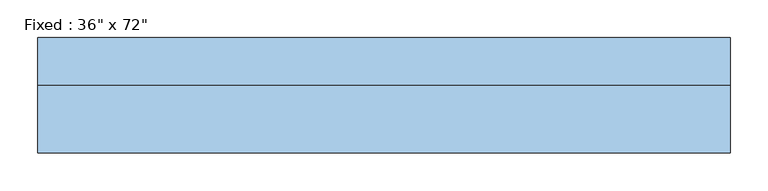
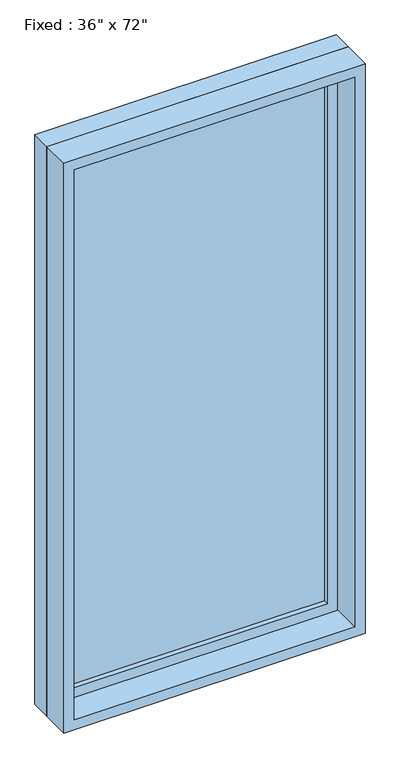
"""IFC4 building model written with IfcOpenShell, lengths in millimetres: window geometry."""

from ifc_helpers import new_model, si_unit, frame, origin, place, context, project, spatial, polyline, outline, extrude, source, transform, mapped, element, save


def window_c05a16fb(model_context):
    return source(origin(), model_context, "Body", "SweptSolid", [
        extrude(outline(polyline([(355.6, 28.575), (-431.8, 28.575), (-431.8, 41.275), (355.6, 41.275), (355.6, 28.575)])), frame((0.0, 0.0, 368.3), z_axis=(0.0, 0.0, 1.0), x_axis=(1.0, 0.0, 0.0)), (0.0, 0.0, 1.0), 1701.8),
        extrude(outline(polyline([(2114.55, -476.25), (323.85, -476.25), (323.85, 400.05), (2114.55, 400.05), (2114.55, -476.25)]), holes=[polyline([(2070.1, -431.8), (2070.1, 355.6), (368.3, 355.6), (368.3, -431.8), (2070.1, -431.8)])]), frame((0.0, 12.7, 0.0), z_axis=(0.0, 1.0, 0.0), x_axis=(0.0, 0.0, 1.0)), (0.0, 0.0, 1.0), 44.45),
        extrude(outline(polyline([(2133.6, -495.3), (304.8, -495.3), (304.8, 419.1), (2133.6, 419.1), (2133.6, -495.3)]), holes=[polyline([(2101.85, -463.55), (2101.85, 387.35), (336.55, 387.35), (336.55, -463.55), (2101.85, -463.55)])]), frame((0.0, -76.2, 0.0), z_axis=(0.0, 1.0, 0.0), x_axis=(0.0, 0.0, 1.0)), (0.0, 0.0, 1.0), 88.9),
        extrude(outline(polyline([(2133.6, 419.1), (2133.6, -495.3), (304.8, -495.3), (304.8, 419.1), (2133.6, 419.1)]), holes=[polyline([(2114.55, 400.05), (323.85, 400.05), (323.85, -476.25), (2114.55, -476.25), (2114.55, 400.05)])]), frame((0.0, 12.7, 0.0), z_axis=(0.0, 1.0, 0.0), x_axis=(0.0, 0.0, 1.0)), (0.0, 0.0, 1.0), 63.5),
    ])


if __name__ == "__main__":
    model = new_model("IFC4")
    model_context = context("Model", 3, world=origin())
    ifc_project = project(units=[si_unit("LENGTHUNIT", "METRE", prefix="MILLI")], contexts=[model_context])
    site = spatial("IfcSite", under=ifc_project)
    building = spatial("IfcBuilding", under=site)
    placement = place(None, origin())
    window_shape = window_c05a16fb(model_context)
    element("IfcWindow", 1, ObjectType="Fixed : 36\" x 72\"", at=placement, inside=building, context=model_context, shape_type="MappedRepresentation", body=[
        mapped(window_shape, transform((0.0, 0.0, 0.0), x_axis=(1.0, 0.0, 0.0), y_axis=(0.0, 1.0, 0.0), z_axis=(0.0, 0.0, 1.0))),
    ])
    save(model, "model.ifc")

# Revit data of these elements
# Type "Fixed : 36\" x 72\""
#   Type Mark = "9"
#   Construction Type Id = "GSP4R"
#   Assembly Code = "B2020100"
#   Analytic Construction = "1/8 in Pilkington single glazing"
#   Visual Light Transmittance = 0.9
#   Solar Heat Gain Coefficient = 0.78
#   Heat Transfer Coefficient (U) = 0.6496 BTU/(h·ft²·°F)
#   Height = 6' - 0"
#   Default Sill Height = 1' - 0"
#   Width = 3' - 0"
#   Window Inset = 0' - 0 3/4"
#   Define Thermal Properties by = 1
#   Glass Pane Material = Glass
#   Sash Material = Sash
#   Wall Closure = (empty or 0)
# Element 1 (IfcWindow, "Fixed : 36\" x 72\"")
#   Materials on its faces: "Sash", "Glass"
# Materials
#   "Glass": class "Glass", colour RGB 0 128 192, transparency 0.75, Description = "Soda Lime Glass", Cost = 0
#   "Sash": class "Wood", colour RGB 224 178 126, transparency 0
